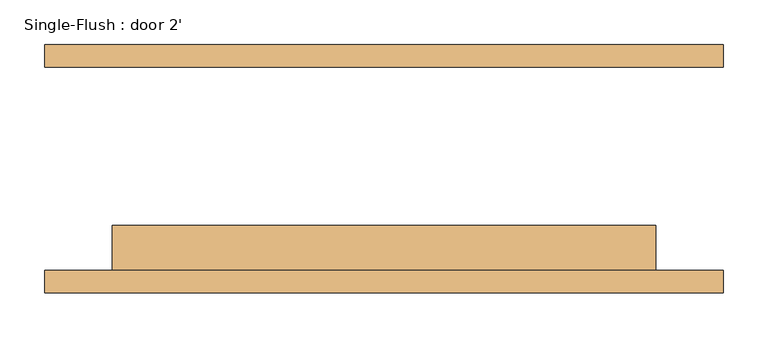
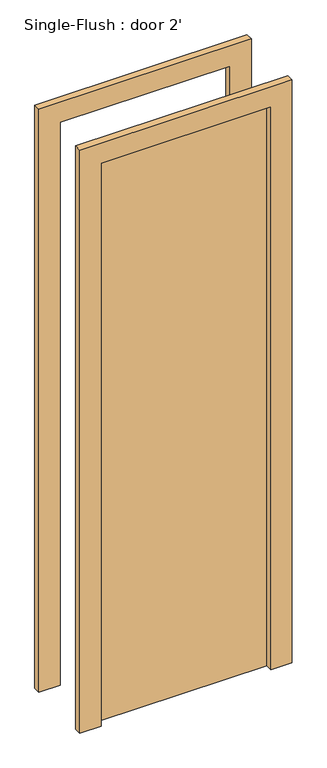
"""IFC4 building model written with IfcOpenShell, lengths in millimetres: door geometry, Single-Flush : door 2'."""

from ifc_helpers import new_model, si_unit, frame, origin, origin_with_axes, place, context, project, spatial, polyline, outline, extrude, source, transform, mapped, element, save


def single_flush_door_2_4a3212df(model_context):
    return source(origin(), model_context, "Body", "SweptSolid", [
        extrude(outline(polyline([(2209.8, -381.0), (0.0, -381.0), (0.0, -304.8), (2133.6, -304.8), (2133.6, 304.8), (0.0, 304.8), (0.0, 381.0), (2209.8, 381.0), (2209.8, -381.0)])), frame((0.0, -139.7, 0.0), z_axis=(0.0, 1.0, 0.0), x_axis=(0.0, 0.0, 1.0)), (0.0, 0.0, 1.0), 25.4),
        extrude(outline(polyline([(2209.8, 381.0), (2209.8, -381.0), (0.0, -381.0), (0.0, -304.8), (2133.6, -304.8), (2133.6, 304.8), (0.0, 304.8), (0.0, 381.0), (2209.8, 381.0)])), frame((0.0, 114.3, 0.0), z_axis=(0.0, 1.0, 0.0), x_axis=(0.0, 0.0, 1.0)), (0.0, 0.0, 1.0), 25.4),
        extrude(outline(polyline([(304.8, -63.5), (304.8, -114.3), (-304.8, -114.3), (-304.8, -63.5), (304.8, -63.5)])), origin_with_axes(), (0.0, 0.0, 1.0), 2133.6),
    ])


if __name__ == "__main__":
    model = new_model("IFC4")
    model_context = context("Model", 3, world=origin())
    ifc_project = project(units=[si_unit("LENGTHUNIT", "METRE", prefix="MILLI")], contexts=[model_context])
    site = spatial("IfcSite", under=ifc_project)
    building = spatial("IfcBuilding", under=site)
    placement = place(None, origin())
    single_flush_door_2_shape = single_flush_door_2_4a3212df(model_context)
    element("IfcDoor", 1, ObjectType="Single-Flush : door 2'", at=placement, inside=building, context=model_context, shape_type="MappedRepresentation", body=[
        mapped(single_flush_door_2_shape, transform((0.0, 0.0, 0.0), x_axis=(1.0, 0.0, 0.0), y_axis=(0.0, 1.0, 0.0), z_axis=(0.0, 0.0, 1.0))),
    ])
    save(model, "model.ifc")

# Revit data of these elements
# Type "Single-Flush : door 2'"
#   Type Mark = "11"
#   Construction Type Id = "MDOOR"
#   Assembly Code = "C1020"
#   Analytic Construction = "Metal"
#   Thickness = 0' - 2"
#   Heat Transfer Coefficient (U) = 0.651978 BTU/(h·ft²·°F)
#   Height = 7' - 0"
#   Trim Projection Ext = 0' - 1"
#   Trim Projection Int = 0' - 1"
#   Trim Width = 0' - 3"
#   Width = 2' - 0"
#   Define Thermal Properties by = 1
#   Door Material = Door - Panel
#   Frame Material = Door - Frame
#   Visual Light Transmittance = 0
#   Solar Heat Gain Coefficient = 0
#   Function = (empty or 0)
#   Wall Closure = (empty or 0)
# Element 1 (IfcDoor, "Single-Flush : door 2'")
#   Materials on its faces: "Door - Frame", "Door - Panel"
# Materials
#   "Door - Panel": class "Wood", colour RGB 210 159 95, transparency 0, Cost = 0
#   "Door - Frame": colour RGB 118 70 51, transparency 0, Cost = 0
